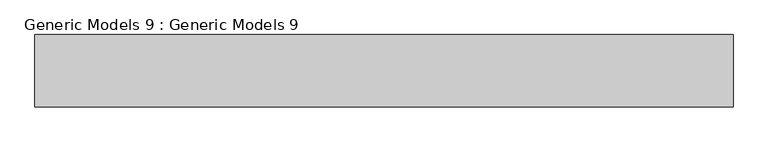
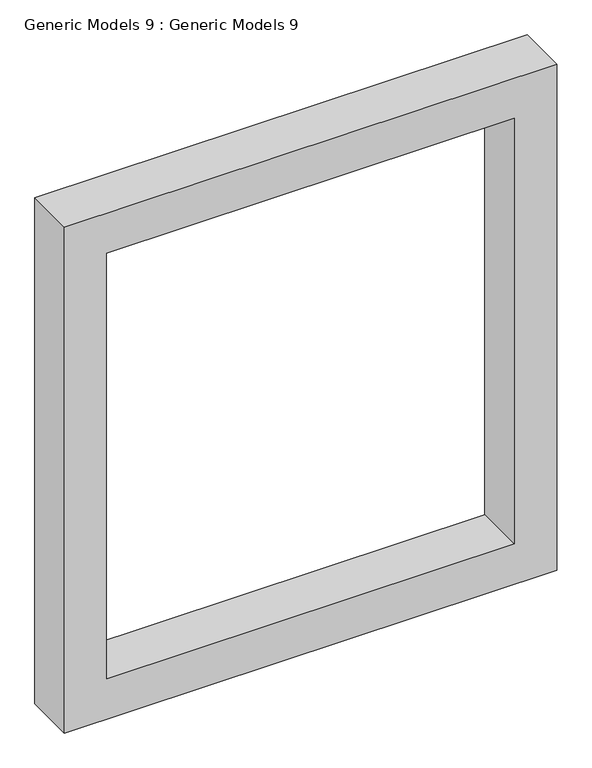
"""IFC4 building model written with IfcOpenShell, lengths in millimetres: proxy geometry, Generic Models 9 : Generic Models 9."""

from ifc_helpers import new_model, si_unit, frame, origin, place, context, project, spatial, polyline, outline, extrude, source, transform, mapped, element, save


def generic_models_9_generic_models_9_4a2afa81(model_context):
    return source(origin(), model_context, "Body", "SweptSolid", [
        extrude(outline(polyline([(2692.4, -3435.4607439), (2692.4, -4908.6607439), (1092.2, -4908.6607439), (1092.2, -3435.4607439), (2692.4, -3435.4607439)]), holes=[polyline([(2565.4, -3562.4607439), (1219.2, -3562.4607439), (1219.2, -4781.6607439), (2565.4, -4781.6607439), (2565.4, -3562.4607439)])]), frame((0.0, -6722.8842658, 0.0), z_axis=(0.0, 1.0, 0.0), x_axis=(0.0, 0.0, 1.0)), (0.0, 0.0, 1.0), 152.4),
    ])


if __name__ == "__main__":
    model = new_model("IFC4")
    model_context = context("Model", 3, world=origin())
    ifc_project = project(units=[si_unit("LENGTHUNIT", "METRE", prefix="MILLI")], contexts=[model_context])
    site = spatial("IfcSite", under=ifc_project)
    building = spatial("IfcBuilding", under=site)
    placement = place(None, origin())
    generic_models_9_generic_models_9_shape = generic_models_9_generic_models_9_4a2afa81(model_context)
    element("IfcBuildingElementProxy", 1, Name="Generic Models 9 : Generic Models 9", ObjectType="Generic Models 9 : Generic Models 9", at=placement, inside=building, context=model_context, shape_type="MappedRepresentation", body=[
        mapped(generic_models_9_generic_models_9_shape, transform((0.0, 0.0, 0.0), x_axis=(1.0, 0.0, 0.0), y_axis=(0.0, 1.0, 0.0), z_axis=(0.0, 0.0, 1.0))),
    ])
    save(model, "model.ifc")

# Revit data of these elements
# Element 1 (IfcBuildingElementProxy, "Generic Models 9 : Generic Models 9")
#   Materials on its faces: "BLACK"
# Materials
#   "BLACK": class "Generic", colour RGB 120 120 120, transparency 0, Cost = 0
